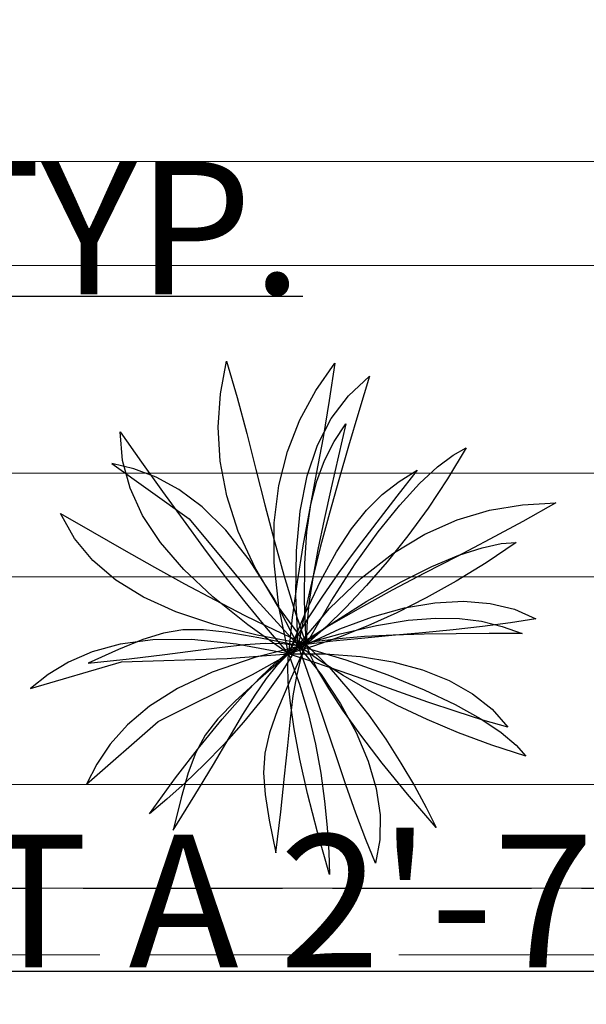
# Model space of a CAD drawing. Units: inches. Extents: x 351 to 1738, y -265 to 286.
# Tile 12 of 38: x 1142 to 1176, y -206 to -147. Entities that reach past the tile are written whole.
import ezdxf

# ---------------------------------------------------------------- set-up
doc = ezdxf.new("R2010")
doc.units = ezdxf.units.IN
doc.header["$MEASUREMENT"] = 0
doc.linetypes.add('ACAD_ISO02W100', pattern=[15, 12, -3])
for name, color, linetype, lineweight in [('A-ANNO-DIMS', 2, 'Continuous', 18), ('A-FLOR-OVHD', 1, 'ACAD_ISO02W100', 18), ('A-FLOR-PATT', 9, 'Continuous', 9)]:
    doc.layers.add(name, color=color, linetype=linetype, lineweight=lineweight)
doc.layers.add('CAY', color=94, linetype='Continuous')
doc.layers.add('DIENHOA', color=3, linetype='Continuous')
doc.styles.get("Standard").update_dxf_attribs({"font": 'arial.ttf'})
doc.dimstyles.get("Standard").update_dxf_attribs({"dimtxt": 8, "dimasz": 5, "dimexe": 0.18, "dimexo": 0.0625, "dimgap": 0.09, "dimtad": 1, "dimtoh": 1, "dimzin": 0, "dimdsep": 46, "dimlunit": 4, "dimtxsty": 'Standard', "dimcen": 0, "dimclre": 256, "dimadec": 0, "dimazin": 0, "dimtfac": 1, "dimtofl": 0, "dimtmove": 0, "dimatfit": 3, "dimfxl": 1, "dimtolj": 1, "dimtzin": 0, "dimlwe": -1, "dimarcsym": 0})

# ---------------------------------------------------------------- blocks, each defined once
blk = doc.blocks.new('Cay03_mb')
at = {"layer": 'DIENHOA'}
for p, q in [((118.6, 555.3), (166.2, 599.1)), ((166.2, 599.1), (142.2, 519.4)), ((79.5, 503.7), (118.6, 555.3)), ((142.2, 519.4), (119, 441.7)), ((48.6, 443.6), (79.5, 503.7)), ((25.5, 374.3), (48.6, 443.6)), ((119, 441.7), (96.7, 365.6)), ((-365.2, 390.3), (-414.4, 402.8)), ((-414.4, 402.8), (-240.2, 277.8)), ((-314.9, 371.3), (-365.2, 390.3)), ((-263.5, 343.5), (-314.9, 371.3)), ((9.9, 295.3), (25.5, 374.3)), ((96.7, 365.6), (75.6, 290.6)), ((-211.2, 304.6), (-263.5, 343.5)), ((511, 309.6), (585.9, 313.5)), ((585.9, 313.5), (511.8, 271.4)), ((-158, 252.3), (-211.2, 304.6)), ((1.6, 205.7), (9.9, 295.3)), ((75.6, 290.6), (55.7, 216.3)), ((363.4, 275.4), (436.8, 297.2)), ((436.8, 297.2), (511, 309.6)), ((-240.2, 277.8), (-88.4, 94.9)), ((290.6, 243.2), (363.4, 275.4)), ((511.8, 271.4), (437.6, 231.5)), ((-104.2, 184.4), (-158, 252.3)), ((218.5, 199.8), (290.6, 243.2)), ((437.6, 231.5), (363.7, 192.9)), ((0.2, 104.9), (1.6, 205.7)), ((55.7, 216.3), (37.3, 142.1)), ((-49.6, 98.5), (-104.2, 184.4)), ((147, 144.1), (218.5, 199.8)), ((363.7, 192.9), (290.2, 154.9)), ((37.3, 142.1), (20.5, 67.6)), ((75.9, 75.2), (147, 144.1)), ((290.2, 154.9), (217.4, 116.6)), ((217.4, 116.6), (145.5, 77.3)), ((-88.4, 94.9), (5.4, -7.8)), ((5.4, -7.8), (-49.6, 98.5)), ((5.4, -7.8), (0.2, 104.9)), ((5.4, -7.8), (75.9, 75.2)), ((20.5, 67.6), (5.4, -7.8)), ((145.5, 77.3), (74.7, 36.1)), ((182.2, 37.2), (253, 48.9)), ((253, 48.9), (314.6, 54.1)), ((314.6, 54.1), (369.2, 53.3)), ((369.2, 53.3), (418.6, 46.8)), ((418.6, 46.8), (464.9, 35.2)), ((-254.7, 27.4), (-298.6, 20.1)), ((-208, 27.8), (-254.7, 27.4)), ((-152.7, 21.7), (-208, 27.8)), ((74.7, 36.1), (5.4, -7.8)), ((100.3, 18.4), (182.2, 37.2)), ((464.9, 35.2), (510, 19)), ((-345, 5.4), (-399.6, -17.1)), ((-298.6, 20.1), (-345, 5.4)), ((-83.4, 9.7), (-152.7, 21.7)), ((5.4, -7.8), (-83.4, 9.7)), ((5.4, -7.8), (100.3, 18.4)), ((46.3, 0.9), (5.4, -7.8)), ((96.7, 7.5), (46.3, 0.9)), ((155, 12.2), (96.7, 7.5)), ((219.6, 15.4), (155, 12.2)), ((289, 17.4), (219.6, 15.4)), ((361.6, 18.5), (289, 17.4)), ((435.8, 18.9), (361.6, 18.5)), ((510, 19), (435.8, 18.9)), ((-399.6, -17.1), (-468, -47.9)), ((-295.3, -27.9), (-225.8, -18.9)), ((-225.8, -18.9), (-165.8, -11.3)), ((-165.8, -11.3), (-114, -5.7)), ((-114, -5.7), (-69, -2.9)), ((-69, -2.9), (-29.6, -3.4)), ((5.4, -7.8), (-33.2, -69.5)), ((-29.6, -3.4), (5.4, -7.8)), ((-16.5, -22.4), (5.4, -7.8)), ((5.4, -7.8), (56.8, -73.3)), ((25.9, -64.4), (5.4, -7.8)), ((5.4, -7.8), (112.8, -40.3)), ((53.5, -41.6), (5.4, -7.8)), ((-468, -47.9), (-375.6, -37.8)), ((-375.6, -37.8), (-295.3, -27.9)), ((-45.1, -46.3), (-16.5, -22.4)), ((107, -75.7), (53.5, -41.6)), ((112.8, -40.3), (207.5, -73.8)), ((-79.8, -79.6), (-45.1, -46.3)), ((47, -125.9), (25.9, -64.4)), ((-120.2, -122.1), (-79.8, -79.6)), ((-33.2, -69.5), (-74.6, -127.3)), ((56.8, -73.3), (100.4, -139.1)), ((165.5, -109.6), (107, -75.7)), ((207.5, -73.8), (289.5, -107.6)), ((228.7, -142.8), (165.5, -109.6)), ((289.5, -107.6), (359.3, -141.1)), ((-165.9, -174.1), (-120.2, -122.1)), ((-74.6, -127.3), (-117.8, -181.1)), ((68.7, -190.6), (47, -125.9)), ((100.4, -139.1), (135.9, -204.3)), ((296, -174.7), (228.7, -142.8)), ((359.3, -141.1), (416.9, -173.5)), ((-216.3, -235.6), (-165.9, -174.1)), ((367.1, -204.8), (296, -174.7)), ((416.9, -173.5), (462.6, -204.2)), ((-117.8, -181.1), (-162.1, -230.9)), ((90.8, -256.6), (68.7, -190.6)), ((135.9, -204.3), (162.8, -268.3)), ((441.6, -232.7), (367.1, -204.8)), ((462.6, -204.2), (496.5, -232.5)), ((-271, -306.6), (-216.3, -235.6)), ((-162.1, -230.9), (-206.3, -276.5)), ((518.9, -257.7), (441.6, -232.7)), ((496.5, -232.5), (518.9, -257.7)), ((113.1, -322.2), (90.8, -256.6)), ((-206.3, -276.5), (-249.6, -317.8)), ((162.8, -268.3), (181, -330.4)), ((-329.5, -387.1), (-271, -306.6)), ((-249.6, -317.8), (-291, -354.7)), ((135.4, -385.6), (113.1, -322.2)), ((181, -330.4), (190, -390)), ((-291, -354.7), (-329.5, -387.1)), ((157.6, -445), (135.4, -385.6)), ((190, -390), (189.6, -446.3)), ((179.5, -498.7), (157.6, -445)), ((189.6, -446.3), (179.5, -498.7))]:
    blk.add_line(p, q, dxfattribs=at)
for points in [[(23.7, -5.4), (-41, 82.2), (-91.8, 167.1), (-129.7, 249.5), (-155.6, 329.6), (-170.2, 407.8), (-174.7, 484.2), (-169.8, 559.3), (-156.5, 633.1)], [(-156.5, 633.1), (-132.5, 551.3), (-110.5, 470), (-89.8, 389.2), (-69.6, 309), (-49, 229.4), (-27.1, 150.4), (-3.2, 72.1), (23.7, -5.4)], [(-16.4, -26.7), (-38.3, 80), (-48.9, 178.3), (-48.7, 269), (-38.5, 352.6), (-19.1, 429.7), (9, 501), (44.9, 567.1), (87.9, 628.5)], [(87.9, 628.5), (75.5, 544.2), (61.3, 461.2), (46.1, 379.1), (30.8, 297.8), (16.1, 216.9), (2.9, 136), (-8.3, 54.9), (-16.4, -26.7)], [(23.7, -5.4), (19.8, 93), (20.3, 177), (25, 248.5), (34, 309.8), (47.3, 362.7), (64.9, 409.3), (86.8, 451.7), (112.9, 491.9)], [(112.9, 491.9), (96, 419.7), (79.5, 347.4), (63.9, 276.5), (50, 208.4), (38.4, 144.8), (29.7, 86.9), (24.6, 36.3), (23.7, -5.4)], [(-395.6, 473.7), (-347.5, 405.6), (-300.6, 339.5), (-254.3, 275.1), (-208.3, 212.3), (-161.9, 150.9), (-114.8, 90.7), (-66.5, 31.6), (-16.4, -26.7)], [(-16.4, -26.7), (-108.3, 38.6), (-186.9, 101.7), (-252.4, 163.5), (-305.1, 224.4), (-345.4, 285.2), (-373.7, 346.6), (-390.4, 409.2), (-395.6, 473.7)], [(384.3, 437.5), (342.2, 367.8), (298.1, 301.7), (252.6, 239.4), (206.1, 181.1), (159.4, 127.2), (113, 78), (67.6, 33.6), (23.7, -5.4)], [(23.7, -5.4), (79.9, 91.7), (134.1, 176.2), (185.8, 248.4), (234.3, 308.7), (279, 357.3), (319.3, 394.8), (354.6, 421.4), (384.3, 437.5)], [(273.2, 387.3), (227.6, 328.8), (182.3, 270.1), (138.4, 212.3), (97.2, 156.4), (60, 103.4), (27.8, 54.6), (1.9, 10.8), (-16.4, -26.7)], [(-16.4, -26.7), (21.4, 64.2), (57, 140.3), (91.4, 203.3), (125.2, 255.1), (159.5, 297.5), (195, 332.5), (232.7, 361.8), (273.2, 387.3)], [(-530.5, 289.7), (-458.3, 248.1), (-387.9, 207.8), (-318.9, 168.7), (-250.8, 131.1), (-182.9, 94.8), (-114.9, 59.9), (-46.2, 26.5), (23.7, -5.4)], [(23.7, -5.4), (-87.2, 15.2), (-185, 39.6), (-270.3, 68.2), (-343.7, 101.4), (-405.9, 139.7), (-457.3, 183.5), (-498.7, 233.4), (-530.5, 289.7)], [(496.7, 224), (429.4, 178.4), (361.6, 136.9), (294.1, 99.5), (227.5, 66.1), (162.4, 36.7), (99.7, 11.5), (39.8, -9.7), (-16.4, -26.7)], [(-16.4, -26.7), (75.4, 37.9), (160.1, 91.8), (237.3, 135.7), (306.6, 170), (367.6, 195.4), (419.9, 212.5), (463.1, 221.9), (496.7, 224)], [(23.7, -5.4), (99.3, 29.7), (173.2, 57.1), (244.8, 76.7), (313.3, 88.3), (377.9, 91.8), (437.9, 87), (492.7, 73.8), (541.4, 52)], [(541.4, 52), (484.1, 42.9), (421.2, 34.8), (354.4, 27.6), (285.4, 20.9), (216.1, 14.5), (148.2, 8.1), (83.5, 1.6), (23.7, -5.4)], [(-16.4, -26.7), (-134, -4.7), (-235.3, 5.3), (-322, 4.7), (-395.9, -5), (-458.7, -22.3), (-512.3, -45.7), (-558.2, -73.6), (-598.4, -104.7)], [(-471.9, -320.3), (-310.5, -179.3), (-97.7, -73.3), (23.7, -5.4)], [(23.7, -5.4), (-92.3, -34.8), (-188.4, -68.2), (-266.9, -105.1), (-329.9, -144.9), (-379.7, -187), (-418.5, -230.7), (-448.5, -275.3), (-471.9, -320.3)], [(23.7, -5.4), (-13.6, -87.9), (-41.1, -152.6), (-59.6, -205), (-69.9, -250.7), (-72.8, -295), (-69.2, -343.6), (-59.7, -401.9), (-45.3, -475.5)], [(-45.3, -475.5), (-34.1, -383.2), (-25.4, -302.8), (-18.3, -233.1), (-12, -172.9), (-5.6, -121.2), (2, -76.8), (11.4, -38.5), (23.7, -5.4)], [(316.5, -418.1), (251.4, -342.8), (194.8, -273.3), (146.5, -210.2), (106.3, -153.8), (74.1, -104.7), (49.7, -63.4), (32.9, -30.1), (23.7, -5.4)], [(23.7, -5.4), (74.9, -57.1), (121.8, -110.6), (164.3, -165), (202.7, -219.4), (237, -272.9), (267.3, -324.5), (293.7, -373.2), (316.5, -418.1)], [(-598.4, -104.7), (-392.7, -44.4), (-155, -37.4), (-16.4, -26.7)], [(-276.2, -424.4), (-227.3, -345.4), (-185.7, -276.1), (-150, -215.7), (-119.1, -163.8), (-91.5, -119.5), (-66, -82.3), (-41.4, -51.6), (-16.4, -26.7)], [(-16.4, -26.7), (-84.9, -86), (-137, -133.1), (-175.8, -173), (-204.3, -210), (-225.5, -249.1), (-242.5, -294.7), (-258.4, -351.6), (-276.2, -424.4)], [(76.2, -524.2), (48.8, -428.5), (26.6, -341.7), (9.2, -264.1), (-3.6, -196.1), (-12.3, -138), (-17.1, -90.2), (-18.3, -53), (-16.4, -26.7)], [(-16.4, -26.7), (66.9, -26.6), (145.6, -32.7), (218.8, -44.9), (285.8, -63.1), (345.9, -87.1), (398.4, -116.6), (442.6, -151.6), (477.6, -191.8)], [(477.6, -191.8), (421.8, -176), (361.3, -156.9), (297.6, -135.5), (232.2, -112.6), (166.6, -89.4), (102.3, -66.6), (40.8, -45.4), (-16.4, -26.7)], [(-16.4, -26.7), (8.5, -95.1), (28.5, -163.3), (44.3, -230.6), (56.3, -296.1), (65, -359), (70.9, -418.5), (74.5, -473.9), (76.2, -524.2)]]:
    blk.add_lwpolyline(points, dxfattribs=at)
blk = doc.blocks.new('*D36')
at = {"layer": 'A-ANNO-DIMS', "transparency": 16777216}
for p, q in [((1073.569, -199.341), (1073.569, -204.202)), ((1105.198, -199.341), (1105.198, -204.202))]:
    blk.add_line(p, q, dxfattribs=at)
at = {"layer": 'A-ANNO-DIMS', "color": 0, "lineweight": -2, "transparency": 16777216}
for p, q in [((1078.569, -204.022), (1100.198, -204.022)), ((1105.198, -204.022), (1227.071, -204.022))]:
    blk.add_line(p, q, dxfattribs=at)
at = {"layer": 'A-ANNO-DIMS', "color": 0, "transparency": 16777216}
for points in [[(1078.569, -203.189), (1078.569, -204.856), (1073.569, -204.022)], [(1100.198, -203.189), (1100.198, -204.856), (1105.198, -204.022)]]:
    blk.add_solid(points, dxfattribs=at)
at = {"layer": 'Defpoints', "color": 0, "transparency": 16777216}
for p in [(1073.569, -199.278), (1105.198, -199.278), (1105.198, -204.022)]:
    blk.add_point(p, dxfattribs=at)
at = {"layer": 'A-ANNO-DIMS', "color": 0, "transparency": 16777216, "insert": (1168.634, -199.796), "char_height": 8, "attachment_point": 5}
blk.add_mtext('\\A1;PLANT A 2\'-7 1/2" TYP.', dxfattribs=at)
blk = doc.blocks.new('*D37')
at = {"layer": 'A-ANNO-DIMS', "color": 0, "lineweight": -2, "transparency": 16777216}
for p, q in [((1109.942, -168.369), (1109.942, -163.369)), ((1109.942, -163.369), (1158.933, -163.369)), ((1109.942, -194.278), (1109.942, -173.369))]:
    blk.add_line(p, q, dxfattribs=at)
at = {"layer": 'A-ANNO-DIMS', "transparency": 16777216}
for p, q in [((1105.26, -168.369), (1110.122, -168.369)), ((1105.26, -199.278), (1110.122, -199.278))]:
    blk.add_line(p, q, dxfattribs=at)
at = {"layer": 'A-ANNO-DIMS', "color": 0, "transparency": 16777216}
for points in [[(1109.109, -173.369), (1110.775, -173.369), (1109.942, -168.369)], [(1109.109, -194.278), (1110.775, -194.278), (1109.942, -199.278)]]:
    blk.add_solid(points, dxfattribs=at)
at = {"layer": 'Defpoints', "color": 0, "transparency": 16777216}
for p in [(1105.198, -168.369), (1109.942, -168.369), (1105.198, -199.278)]:
    blk.add_point(p, dxfattribs=at)
at = {"layer": 'A-ANNO-DIMS', "color": 0, "transparency": 16777216, "insert": (1134.482, -159.26), "char_height": 8, "attachment_point": 5}
blk.add_mtext('\\A1;2\'-7" TYP.', dxfattribs=at)

msp = doc.modelspace()

# ---------------------------------------------------------------- hatches: boundary and pattern name
at = {"layer": 'A-FLOR-PATT', "transparency": 33554559}
h = msp.add_hatch(dxfattribs=at)
h.set_pattern_fill('ANSI37', color=256, scale=200, angle=135)
h.set_pattern_definition([(180, (1112.704, -164.037), (-2e-15, -25), []), (270, (1112.704, -164.037), (25, -5e-15), [])])
h.paths.add_polyline_path([(1380.064, 73.463), (1380.132, 148.463), (1338.064, 148.463), (1290.704, 148.463), (1290.704, 88.463), (1248.704, 88.463), (1248.704, -2.009), (1244.704, -2.009), (1244.704, 142.457), (1160.704, 142.457), (1160.704, 158.963), (1160.704, 170.137), (1160.704, 206.137), (1160.704, 228.963), (1112.704, 228.963), (1112.704, 209.963), (1112.704, 168.963), (1124.704, 168.963), (1124.704, 162.963), (1112.704, 162.963), (1112.704, 64.463), (1112.704, 60.463), (1112.704, 0.463), (1112.704, -48.026), (1146.804, -47.981), (1146.804, -35.691), (1207.804, -35.691), (1207.804, -47.902), (1236.542, -47.864), (1236.544, -50.009), (1248.5, -50.009), (1248.506, -102.915), (1248.512, -150.915), (1248.514, -164.037), (1248.549, -164.037), (1273.017, -164.037), (1273.017, -128.799), (1355.24, -128.799), (1355.24, -164.037), (1384.204, -164.037), (1384.204, -57.037), (1380.064, -57.037), (1380.064, -48.037), (1392.064, -48.037), (1392.064, -53.037), (1406.549, -53.037), (1406.549, -57.037), (1401.204, -57.037), (1401.204, -147.037), (1468.204, -147.037), (1468.204, -138.5), (1472.204, -138.5), (1472.204, -102.5), (1468.204, -102.5), (1468.204, -57.037), (1442.549, -57.037), (1442.549, -53.037), (1463.049, -53.037), (1463.049, -40.747), (1524.049, -40.747), (1524.049, -48.037), (1536.064, -48.037), (1536.064, -53.037), (1557.704, -53.037), (1557.704, 204.963), (1384.204, 204.963), (1384.204, 73.463), (1392.064, 73.463), (1392.064, 64.463), (1384.204, 64.463), (1384.204, -3.5), (1380.204, -3.537), (1380.204, 64.463), (1380.064, 64.463)])
h.paths.add_polyline_path([(1510.714, 86.458, -0.103984), (1511.661, 85.595, 0.470438), (1510.158, 87.614, 0.0961)], flags=16)
h.paths.add_polyline_path([(1510.443, 100.266, 0.009798), (1504.693, 100.48, 0.02879), (1504.6, 99.767, -0.165331), (1505.519, 96.135, -0.143601)], flags=16)
h.paths.add_polyline_path([(1487.201, 85.595, -0.103984), (1488.148, 86.458, 0.0961), (1488.704, 87.614, 0.470438)], flags=0)
h.paths.add_polyline_path([(1495.052, 100.43), (1494.178, 100.43, -0.026463), (1494.262, 99.774, -0.144219)], flags=16)
h.paths.add_polyline_path([(1444.485, 86.458, -0.103984), (1445.433, 85.595, 0.470438), (1443.93, 87.614, 0.0961)], flags=16)
h.paths.add_polyline_path([(1420.972, 85.595, -0.103984), (1421.92, 86.458, 0.0961), (1422.475, 87.614, 0.470438)], flags=16)
h.paths.add_polyline_path([(1428.632, 100.335, 0.001054), (1427.971, 100.309, -0.021524), (1428.033, 99.774, -0.114301)], flags=16)
h.paths.add_polyline_path([(1419.906, 143.708, 0.024979), (1420.222, 157.526), (1421.573, 159.101), (1421.573, 175.369), (1391.393, 175.369), (1391.393, 200.519), (1542.294, 200.519), (1542.294, 175.369), (1512.028, 175.369, 0.019865), (1511.521, 153.838, 0.025134), (1512.758, 118.323, 0.020553), (1512.942, 115.253), (1419.834, 115.253, -0.000414), (1419.843, 124.798), (1413.059, 124.798), (1413.059, 84.437, -0.061853), (1415.831, 80.45, -0.093077), (1420.972, 85.595, -0.267537), (1422.371, 84.732, 0.08511), (1424.052, 84.616, -0.885393), (1424.033, 84.851, -1.125815), (1424.073, 84.366, -0.087987), (1422.371, 84.732, -0.267537), (1422.326, 83.089, -0.370542), (1420.972, 85.595, 0.093077), (1415.831, 80.45, -0.087414), (1417.914, 73.937), (1418.941, 73.937, 0.02725), (1418.913, 76.906, -0.115703), (1421.051, 73.937), (1445.354, 73.937, -0.115703), (1447.492, 76.906, 0.02725), (1447.464, 73.937), (1448.491, 73.937, -0.087414), (1450.574, 80.45, 0.093077), (1445.433, 85.595, -0.370542), (1444.079, 83.089, -0.267537), (1444.034, 84.732, -0.087987), (1442.332, 84.366, -1.125815), (1442.372, 84.851, -2.032736), (1442.364, 84.368, 0.086378), (1444.034, 84.732, -0.267537), (1445.433, 85.595, -0.093077), (1450.574, 80.45, -0.257732), (1466.483, 90.927, -0.47867), (1468.832, 91.907, -0.47867), (1471.18, 90.927, -0.26264), (1483.053, 81.78, -0.071866), (1487.201, 85.595, -0.267537), (1488.6, 84.732, 0.08511), (1490.28, 84.616, -0.885393), (1490.262, 84.851, -1.125815), (1490.301, 84.366, -0.087987), (1488.6, 84.732, -0.267537), (1488.554, 83.089, -0.370542), (1487.201, 85.595, 0.071866), (1483.053, 81.78, -0.132065), (1484.143, 73.937), (1485.169, 73.937, 0.02725), (1485.142, 76.906, -0.115703), (1487.28, 73.937), (1511.582, 73.937, -0.115703), (1513.72, 76.906, 0.02725), (1513.693, 73.937), (1514.719, 73.937, -0.087414), (1516.802, 80.45, 0.093077), (1511.661, 85.595, -0.370542), (1510.308, 83.089, -0.267537), (1510.262, 84.732, -0.087987), (1508.561, 84.366, -1.125815), (1508.601, 84.851, -2.032736), (1508.592, 84.368, 0.086378), (1510.262, 84.732, -0.267537), (1511.661, 85.595, -0.093077), (1516.802, 80.45, -0.061853), (1519.575, 84.437), (1519.575, 73.937), (1413.059, 73.937), (1413.059, 124.798), (1419.843, 124.798, -0.000821)], flags=16)
h.paths.add_polyline_path([(1220.149, 54.133, -0.103984), (1220.869, 53.476, 0.470438), (1219.727, 55.011, 0.0961)], flags=16)
h.paths.add_polyline_path([(1219.944, 64.626, 0.009798), (1215.574, 64.789, 0.02879), (1215.503, 64.247, -0.165331), (1216.201, 61.487, -0.143601)], flags=16)
h.paths.add_polyline_path([(1209.779, 64.449, 0.097446), (1209.339, 64.751), (1208.247, 64.751, 0.12739), (1207.7, 64.326, 0.171586), (1206.95, 61.475, -0.158854), (1207.636, 59.45, 0.015898), (1207.795, 59.218, 0.061546), (1208.598, 59.616, 0.175416), (1208.638, 60.099, -0.284779), (1209.348, 62.472, 0.326216)], flags=16)
h.paths.add_polyline_path([(1169.818, 54.133, -0.103984), (1170.538, 53.476, 0.470438), (1169.396, 55.011, 0.0961)], flags=16)
h.paths.add_polyline_path([(1159.017, 62.472, 0.284764), (1158.307, 60.099, -0.175433), (1158.267, 59.616, 0.39293), (1159.448, 64.449, -0.32623)], flags=16)
h.paths.add_polyline_path([(1156.342, 58.239, -0.178321), (1154.011, 55.31, -0.174736), (1154.722, 55.233, -0.200802), (1156.27, 56.086, 0.12699), (1157.283, 58.991, -0.091205)], flags=16)
h.paths.add_polyline_path([(1156.624, 61.413, 0.157275), (1157.316, 64.247, 0.169622)], flags=16)
h.paths.add_polyline_path([(1152.67, 54.133, -0.0961), (1151.95, 53.476, 0.064076), (1154.465, 54.384, 0.199016)], flags=16)
h.paths.add_polyline_path([(1202.281, 53.476, -0.103984), (1203, 54.133, 0.0961), (1203.423, 55.011, 0.470438)], flags=0)
h.paths.add_polyline_path([(1151.139, 97.64, 0.024979), (1151.379, 108.141), (1152.406, 109.338), (1152.406, 121.701), (1129.47, 121.701), (1129.47, 140.814), (1244.149, 140.814), (1244.149, 121.701), (1221.148, 121.701, 0.019865), (1220.763, 105.338, 0.025134), (1221.703, 78.349, 0.020553), (1221.843, 76.016), (1151.078, 76.016, -0.128743), (1148.786, 65.037, 0.539352), (1150.327, 64.171, -0.027594), (1163.481, 64.751, 0.097695), (1163.04, 64.449, 0.326216), (1163.471, 62.472, -0.284777), (1164.181, 60.099, -0.194757), (1165.846, 61.443, -0.155402), (1165.172, 64.247, -0.166022), (1165.869, 61.475, -0.177014), (1167.852, 62.77, -0.448203), (1169.974, 60.807, -0.393499), (1167.679, 57.86, -0.895548), (1168.438, 54.524, -0.355767), (1166.218, 56.086, -0.066024), (1165.505, 57.539), (1165.251, 56.243, -0.371732), (1164.02, 59.758, -0.373614), (1163.04, 64.449, -0.097695), (1163.481, 64.751, 0.021354), (1153.294, 64.429, -0.134183), (1156.695, 61.368, 0.186873), (1154.636, 62.77, 0.448203), (1152.514, 60.807, 0.403726), (1154.905, 57.846, 0.711219), (1153.334, 55, 0.53154), (1151.95, 53.476, -0.267537), (1153.013, 52.821, 0.08511), (1154.29, 52.732, -0.885393), (1154.276, 52.911, -1.125815), (1154.306, 52.543, -0.087987), (1153.013, 52.821, -0.267537), (1152.978, 51.572, -0.370542), (1151.95, 53.476, 0.093077), (1148.043, 49.566, -0.087414), (1149.626, 44.617), (1150.406, 44.617, 0.02725), (1150.385, 46.873, -0.115703), (1152.01, 44.617), (1170.478, 44.617, -0.115703), (1172.103, 46.873, 0.02725), (1172.082, 44.617), (1172.862, 44.617, -0.087414), (1174.445, 49.566, 0.093077), (1170.538, 53.476, -0.370542), (1169.51, 51.572, -0.267537), (1169.475, 52.821, -0.087987), (1168.182, 52.543, -1.125815), (1168.212, 52.911, -2.032736), (1168.206, 52.544, 0.086378), (1169.475, 52.821, -0.267537), (1170.538, 53.476, -0.093077), (1174.445, 49.566, -0.257732), (1186.536, 57.528, -0.47867), (1188.321, 58.273, -0.47867), (1190.106, 57.528, -0.26264), (1199.128, 50.577, -0.071866), (1202.281, 53.476, -0.267537), (1203.344, 52.821, 0.08511), (1204.621, 52.732, -0.885393), (1204.607, 52.911, -1.125815), (1204.637, 52.543, -0.087987), (1203.344, 52.821, -0.267537), (1203.309, 51.572, -0.370542), (1202.281, 53.476, 0.071866), (1199.128, 50.577, -0.132065), (1199.957, 44.617), (1200.737, 44.617, 0.02725), (1200.716, 46.873, -0.115703), (1202.341, 44.617), (1220.809, 44.617, -0.115703), (1222.434, 46.873, 0.02725), (1222.413, 44.617), (1223.193, 44.617, -0.087414), (1224.776, 49.566, 0.093077), (1220.869, 53.476, -0.370542), (1219.841, 51.572, -0.267537), (1219.806, 52.821, -0.087987), (1218.513, 52.543, -1.125815), (1218.543, 52.911, -2.032736), (1218.537, 52.544, 0.086378), (1219.806, 52.821, -0.267537), (1220.869, 53.476, -0.093077), (1224.776, 49.566, -0.061853), (1226.883, 52.597), (1226.883, 44.617), (1145.936, 44.617), (1145.936, 83.269), (1151.091, 83.269, -0.000821)], flags=16)
h.paths.add_polyline_path([(1218.01, 57.86, -0.895548), (1218.769, 54.524, -0.355767), (1216.549, 56.086, -0.066024), (1215.836, 57.539), (1215.582, 56.243, -0.371732), (1214.351, 59.758, -0.373614), (1213.371, 64.449, 0.326216), (1213.802, 62.472, -0.284777), (1214.512, 60.099, -0.194757), (1216.177, 61.443, -0.179991), (1218.183, 62.77, -0.448203), (1220.305, 60.807, -0.393499)], flags=16)
h.paths.add_polyline_path([(1424.735, 91.363, -0.393499), (1421.715, 95.241, -0.448203), (1424.507, 97.824, -0.179991), (1427.147, 96.077, -0.194757), (1429.338, 94.309, -0.284777), (1430.272, 97.432, 0.326216), (1430.839, 100.034, -0.373614), (1429.55, 93.861, -0.371732), (1427.929, 89.235), (1427.596, 90.941, -0.066024), (1426.657, 89.029, -0.355767), (1423.736, 86.973, -0.895548)], flags=16)
h.paths.add_polyline_path([(1238.033, 131.257, -1), (1227.329, 131.257, -1)], flags=0)
h.paths.add_polyline_path([(1235.357, 131.257, -1), (1230.005, 131.257, -1)], flags=0)
h.paths.add_polyline_path([(1214.039, 54.243, 0.154382), (1214.38, 53.992, 0.358955), (1213.613, 54.016, 0.603948), (1214.379, 53.657, 0.371319), (1213.968, 52.872, 0.187994), (1214.312, 52.809, -0.592455), (1213.953, 52.967, -0.294279), (1214.083, 53.691, -1.300187), (1213.881, 54.134, -0.283762), (1214.469, 53.896, 1.15094)], flags=16)
h.paths.add_polyline_path([(1212.091, 56.286, -0.408434), (1211.337, 56.445, -0.036259), (1211.098, 56.848, -0.236098), (1211.59, 56.63, 0.035345), (1211.835, 56.543, -0.475241), (1212.091, 56.286, -0.475241), (1212.438, 56.182, 0.035345), (1212.631, 56.007, -0.236098), (1213.056, 55.676, -0.036259), (1212.588, 55.697, -0.408434)], flags=16)
h.paths.add_polyline_path([(1211.469, 50.297, 0.296043), (1210.47, 50.527, 0.310883), (1211.931, 50.148, 0.021255)], flags=16)
h.paths.add_polyline_path([(1213.739, 51.818, -0.036259), (1213.271, 51.838, -0.408434), (1212.774, 52.427, -0.094786), (1212.293, 50.703, 1.150474), (1212.911, 50.232, 0.166288), (1213.265, 50.68, -0.025254), (1212.603, 50.13, 1.087932), (1212.471, 49.407, 0.166288), (1213.02, 49.251, -0.016128), (1212.567, 49.563, -0.286859), (1212.217, 49.638, 0.022156), (1212.046, 50.055, -0.64613), (1212.185, 50.498, 0.088412), (1212.732, 52.077, -1.186037), (1213.121, 52.323, 0.035345), (1213.314, 52.148, -0.236098)], flags=16)
h.paths.add_polyline_path([(1212.094, 50.342, -0.048524), (1211.54, 49.605, -1.103834), (1211.397, 48.738, -0.785515), (1211.683, 48.254, -0.392043), (1210.948, 48.525, -0.392819), (1210.561, 47.995, -0.592455), (1210.201, 48.153, -0.294279), (1210.331, 48.877, -0.704172), (1210.316, 49.592, -0.679344), (1210.729, 50.112, 0.563676)], flags=16)
h.paths.add_polyline_path([(1211.274, 49.829, -0.139826), (1210.745, 49.859, -0.217879), (1210.948, 49.509, -0.498572)], flags=0)
h.paths.add_polyline_path([(1433.426, 81.49, -0.181571), (1434.245, 81.788, -0.008067), (1433.726, 82.205, 0.045578), (1432.755, 81.242, 0.179011)], flags=16)
h.paths.add_polyline_path([(1434.146, 81.009, -0.132442), (1433.645, 80.771, 0.259089), (1433.234, 80.471, -0.180211), (1433.392, 80.805, -0.16994), (1432.758, 81.109, 0.032652), (1433.273, 80.474, -0.493363), (1434.046, 80.146, -0.390497)], flags=16)
h.paths.add_polyline_path([(1434.83, 80.047, -0.947538), (1435.294, 79.576, -0.299128), (1434.625, 79.404, -0.270439), (1435.01, 78.591, -0.592455), (1434.537, 78.382, -0.392819), (1434.027, 79.08, -0.392043), (1433.06, 78.723, -0.352042), (1433.003, 79.197, -0.197216), (1433.75, 79.734, -0.71364), (1434.447, 79.939, -0.21479), (1434.819, 80.475, 0.408833), (1435.075, 80.803, -0.226152)], flags=16)
h.paths.add_polyline_path([(1432.67, 81.217, -0.454218), (1431.897, 79.923, -0.414411), (1431.301, 80.035, 0.016129), (1431.897, 80.445, 0.27957), (1432.073, 80.871, -0.289504), (1431.103, 81.321, -0.414411), (1430.978, 81.915, 0.01613), (1431.586, 81.521, 0.341293), (1432.125, 81.583, -0.813186)], flags=16)
h.paths.add_polyline_path([(1429.893, 86.381, -0.947538), (1430.358, 85.91, -0.173106), (1429.984, 85.712, -0.038817), (1431.625, 84.214, -0.0879), (1432.097, 88.549, -0.049768), (1431.254, 88.49, -0.236098), (1431.814, 88.925, 0.035345), (1432.067, 89.155, -0.475241), (1432.524, 89.291, -0.475241), (1432.86, 89.63, 0.035345), (1433.182, 89.744, -0.236098), (1433.83, 90.032, -0.036259), (1433.516, 89.502, -0.408434), (1432.524, 89.291, -0.312424), (1432.106, 88.58, 0.088559), (1431.625, 84.214, -0.408434), (1430.971, 83.439, -0.036259), (1430.355, 83.412, -0.236098), (1430.914, 83.847, 0.035345), (1431.168, 84.078, -0.475241), (1431.625, 84.214, 0.038817), (1429.984, 85.712, -0.321732), (1429.333, 86.048, -0.32743), (1429.883, 86.809, 0.408833), (1430.138, 87.138, -0.226152)], flags=16)
h.paths.add_polyline_path([(1211.206, 58.616, -0.999784), (1211.336, 59.323, -0.614994)], flags=16)
h.paths.add_polyline_path([(1210.288, 49.429, 0.154382), (1210.629, 49.178, 0.358955), (1209.861, 49.202, 0.603948), (1210.627, 48.843, -0.534825), (1210.806, 49.295, 0.748346)], flags=16)
h.paths.add_polyline_path([(1209.589, 51.828, -0.008791), (1209.775, 51.753, 0.112231), (1209.466, 52.019, 1.418851), (1209.014, 51.708, -0.458726), (1208.651, 51.073, -0.592455), (1208.291, 51.232, -0.294279), (1208.421, 51.955, -1.300187), (1208.219, 52.398, -0.226005), (1208.719, 52.257, -0.475519), (1209.158, 52.369, -1.455499), (1209.603, 52.664, 0.421305), (1209.191, 52.262, -0.591212), (1208.979, 51.796, 0.497399), (1209.773, 51.333, 0.649312)], flags=16)
h.paths.add_polyline_path([(1208.029, 52.041, 0.544667), (1208.832, 52.045, 0.220132)], flags=0)
h.paths.add_polyline_path([(1210.438, 51.425, -0.2042), (1210.277, 52.018, 0.270826), (1209.915, 52.897, 0.324115)], flags=0)
h.paths.add_polyline_path([(1209.668, 52.407, -0.60139), (1208.99, 52.221, -0.394916), (1208.248, 52.83, -0.836792), (1208.651, 53.017, -0.338488), (1209.039, 52.571, 0.194138), (1209.191, 52.262, 0.413995), (1209.712, 52.475, 0.51771), (1210.503, 51.416, 0.401922), (1209.493, 50.93, 0.206396), (1209.516, 50.165, -0.319463), (1210.417, 51.418, -0.466635)], flags=16)
h.paths.add_polyline_path([(1206.601, 56.086, -0.355767), (1204.381, 54.524, -0.921198), (1205.236, 57.846, 0.206569), (1207.614, 58.991, -0.12699)], flags=16)
h.paths.add_polyline_path([(1435.487, 82.816, 0.527765), (1436.615, 83.361, 0.50854), (1437.05, 82.433, 0.592455), (1437.524, 82.641, 0.331245), (1436.963, 83.548, 0.387863), (1437.808, 83.626, 0.592954), (1437.618, 84.176, 0.226016), (1436.961, 83.99, 0.318205), (1437.588, 84.854, 0.689374), (1437.05, 84.991, 0.335765), (1436.539, 84.41, -0.156993), (1436.404, 84.065, -0.434611), (1436.961, 83.99, -0.21479), (1437.333, 84.526, 0.408833), (1437.588, 84.854, -0.226152), (1437.343, 84.097, -0.947538), (1437.808, 83.626, -0.299128), (1437.139, 83.455, -0.270439), (1437.524, 82.641, -0.592455), (1437.05, 82.433, -0.392819), (1436.541, 83.13, -0.43966), (1435.475, 82.794, -0.174614), (1435.942, 82.244, -0.206396), (1435.912, 81.237, -0.270826), (1435.125, 82.208, 0.207976), (1434.686, 82.904, -0.196495)], flags=16)
h.paths.add_polyline_path([(1435.386, 84.832, 0.270811), (1434.91, 83.676, -0.204217), (1434.699, 82.895, 0.324115)], flags=0)
h.paths.add_polyline_path([(1435.68, 84.18, -0.217656), (1435.554, 83.304, -0.176705), (1436.236, 83.778, -0.373036)], flags=0)
h.paths.add_polyline_path([(1435.566, 100.034, 0.326216), (1436.133, 97.432, -0.284777), (1437.067, 94.309, -0.194757), (1439.258, 96.077, -0.155402), (1438.371, 99.767, -0.166022), (1439.289, 96.12, -0.177014), (1441.897, 97.824, -0.448203), (1444.69, 95.241, -0.393499), (1441.67, 91.363, -0.895548), (1442.669, 86.973, -0.355767), (1439.748, 89.029, -0.066024), (1438.809, 90.941), (1438.476, 89.235, -0.371732), (1436.855, 93.861, -0.373614)], flags=16)
h.paths.add_polyline_path([(1191.252, 49.507, -0.274022), (1190.658, 48.409, 0.267537), (1191.311, 47.344, 0.370542)], flags=0)
h.paths.add_polyline_path([(1190.301, 49.717, 0.199016), (1188.619, 49.04, 0.064076), (1191.252, 49.507, -0.0961)], flags=0)
h.paths.add_polyline_path([(1189.518, 47.857, 1.125815), (1189.676, 47.523, 2.044605)], flags=0)
h.paths.add_polyline_path([(1464.974, 80.372, 0.274022), (1465.756, 78.927, -0.083013)], flags=0)
h.paths.add_polyline_path([(1464.974, 80.372, 0.370542), (1464.897, 77.525, 0.576324)], flags=0)
h.paths.add_polyline_path([(1464.974, 80.372, -0.470438), (1467.284, 81.372, -0.0961), (1466.226, 80.648, -0.199016), (1468.439, 79.757, -0.064076)], flags=0)
h.paths.add_polyline_path([(1189.511, 56.43, -0.259467), (1188.321, 56.391, -0.259467), (1187.13, 56.43, 0.08511), (1188.193, 55.716, -0.885393), (1188.27, 55.878, -1.196013), (1188.355, 55.442, 0.101459)], flags=0)
h.paths.add_polyline_path([(1188.321, 57.596, 0.078072), (1187.678, 57.24, 0.01555), (1188.321, 57.136, 0.01555), (1188.964, 57.24, 0.078072)], flags=0)
h.paths.add_polyline_path([(1190.164, 55.365, -0.576324), (1190.106, 57.528, -0.198294), (1188.321, 58.319, -0.198294), (1186.536, 57.528, -0.576324), (1186.477, 55.365, -0.370542), (1186.536, 57.528, 0.198294), (1188.321, 58.319, 0.198294), (1190.106, 57.528, -0.370542)], flags=0)
h.paths.add_polyline_path([(1188.372, 55.878, 1.125814), (1188.529, 55.544, 2.044605)], flags=0)
h.paths.add_polyline_path([(1186.341, 49.717, -0.0961), (1185.389, 49.507, 0.064076), (1188.022, 49.04, 0.199016)], flags=0)
h.paths.add_polyline_path([(1185.389, 49.507, -0.267537), (1185.984, 48.409, 0.08511), (1187.046, 47.695, -0.885393), (1187.123, 47.857, -1.125815), (1186.966, 47.523, -0.087987), (1185.984, 48.409, -0.267537), (1185.331, 47.344, -0.370542)], flags=0)
h.paths.add_polyline_path([(1399.441, 187.944, -1), (1413.525, 187.944, -1)], flags=0)
h.paths.add_polyline_path([(1402.962, 187.944, -1), (1410.004, 187.944, -1)], flags=0)
h.paths.add_polyline_path([(1357.663, -72.245), (1377.272, -72.245), (1377.272, -91.854), (1357.663, -91.854)], flags=16)
h.paths.add_polyline_path([(1467.256, 78.201, -1.125815), (1467.049, 77.761, -2.044605)], flags=0)
h.paths.add_polyline_path([(1468.822, 88.714, 0.941125), (1469.106, 88.316, 1.137152), (1468.765, 88.755, 0.890986), (1468.99, 88.245, 0.094828), (1470.398, 89.481, -0.267537), (1471.18, 90.927, -0.028123), (1469.678, 90.547, -0.028774), (1469.948, 90.311, -0.020327), (1468.832, 90.41, -0.020327), (1467.716, 90.311, -0.028774), (1467.986, 90.547, -0.028123), (1466.483, 90.927, -0.267537), (1467.265, 89.481, 0.08511), (1468.663, 88.542, -1.202316)], flags=0)
h.paths.add_polyline_path([(1178.25, 124.523, -0.119929), (1165.65, 124.145, -0.107349), (1159.133, 124.446, -0.102891), (1159.132, 130.465, -0.074897), (1158.993, 137.956, 0.002027), (1167.844, 137.479, -0.07553), (1180.337, 137.666, -0.075861), (1186.502, 137.688, -0.14099), (1186.272, 130.046, -0.095481), (1186.729, 124.748, -0.10603)], flags=0)
h.paths.add_polyline_path([(1469.225, 79.757, -0.199016), (1471.437, 80.648, -0.0961), (1470.379, 81.372, -0.470438), (1472.689, 80.372, -0.370542), (1472.766, 77.525, -0.267537), (1471.907, 78.927, -0.087986), (1470.615, 77.761, -1.125849), (1470.408, 78.201, -2.032736), (1470.642, 77.778, 0.086378), (1471.907, 78.927, -0.267537), (1472.689, 80.372, -0.064076)], flags=0)
h.paths.add_polyline_path([(1430.423, 186.902, -0.074897), (1430.24, 196.758, 0.002027), (1441.887, 196.131, -0.07553), (1458.326, 196.377, -0.075861), (1466.438, 196.406, -0.14099), (1466.136, 186.35, -0.095481), (1466.737, 179.378, -0.10603), (1455.58, 179.082, -0.119929), (1439, 178.585, -0.107349), (1430.425, 178.981, -0.102891)], flags=0)
h.paths.add_polyline_path([(1162.258, 49.939, 0.335765), (1161.87, 49.497, -0.156994), (1161.767, 49.235, -0.434611), (1162.19, 49.178, -0.21479), (1162.473, 49.585, 1.529195)], flags=16)
h.paths.add_polyline_path([(1161.683, 49.021, 0.581518), (1161.268, 49.583, 0.592761)], flags=16)
h.paths.add_polyline_path([(1162.602, 48.058, 0.371319), (1162.192, 48.843, 0.434533), (1162.88, 48.962, 0.185081), (1162.197, 48.926, 1.121837)], flags=16)
h.paths.add_polyline_path([(1161.443, 48.941, -1.307104), (1161.495, 48.571, -0.217752), (1161.136, 48.254, 0.697303), (1161.871, 49.048, 0.121514)], flags=16)
h.paths.add_polyline_path([(1162.531, 49.429, -0.207084), (1162.05, 49.146, -0.99203)], flags=16)
h.paths.add_polyline_path([(1161.304, 49.578, -0.719667), (1161.513, 50.079, -0.130428), (1160.836, 50.168, 0.039593)], flags=0)
h.paths.add_polyline_path([(1162.036, 50.584, -0.008067), (1161.642, 50.9, 0.029367), (1161.35, 50.297, -0.205788)], flags=16)
h.paths.add_polyline_path([(1162.882, 51.392, -0.124733), (1162.763, 51.828, -0.101191), (1162.399, 51.438, -0.153425)], flags=0)
h.paths.add_polyline_path([(1164.235, 51.85, -0.309107), (1164.513, 51.136, -0.627125), (1163.781, 51.603, -0.685909), (1162.777, 51.219, -0.233285), (1163.303, 50.165, -0.270826), (1162.705, 50.903, 0.2042), (1162.381, 51.425, 0.204182), (1162.542, 52.018, -0.270841), (1162.903, 52.897, -0.127261), (1163.219, 52.529, -1.168681), (1163.781, 52.587, -0.329112), (1164.168, 53.017, -0.836792), (1164.571, 52.83, -0.193341), (1164.391, 52.338, -0.947538), (1164.744, 51.981, -0.299128)], flags=16)
h.paths.add_polyline_path([(1163.598, 51.937, -1.262956), (1163.236, 51.831, 0.012575), (1162.971, 51.721, 0.230657), (1163.151, 52.407, -0.164898), (1163.178, 52.661, -0.44932), (1163.628, 52.262, -0.721477), (1164.154, 52.088, -0.849998)], flags=0)
h.paths.add_polyline_path([(1161.613, 58.616, -0.980413), (1161.525, 59.049, -2.908935)], flags=16)
h.paths.add_polyline_path([(1160.252, 49.166, -0.414411), (1159.799, 49.251, 0.016129), (1160.252, 49.563, 0.27957), (1160.386, 49.887, -0.289504), (1159.649, 50.229, -0.414411), (1159.554, 50.68, 0.01613), (1160.015, 50.381, 0.617885), (1160.526, 50.703, -0.094786), (1160.045, 52.427, -0.140444), (1159.682, 52.042, -0.057856), (1159.3, 51.872, 0.544843), (1160.046, 52.419, -0.088122), (1160.404, 55.721, -0.049768), (1159.763, 55.676, -0.236098), (1160.188, 56.007, 0.035345), (1160.381, 56.182, -0.475241), (1160.728, 56.286, -0.475241), (1160.984, 56.543, 0.035345), (1161.229, 56.63, -0.236098), (1161.721, 56.848, -0.036259), (1161.482, 56.445, -0.408434), (1160.728, 56.286, -0.312424), (1160.411, 55.745, 0.088559), (1160.045, 52.427, 0.107081), (1160.634, 50.498, -0.494798), (1160.839, 50.149, -0.454218)], flags=16)
h.paths.add_polyline_path([(1160.666, 49.808, -2.076528), (1160.828, 50.172, 0.019586)], flags=0)
h.paths.add_polyline_path([(1158.439, 53.992, 0.154382), (1158.78, 54.243, 0.748346), (1158.262, 54.109, -0.338225), (1158.492, 53.839, -0.170816), (1159.124, 53.779, 0.495729), (1158.938, 54.134, 0.226016)], flags=16)
h.paths.add_polyline_path([(1160.045, 52.427, 0.038817), (1158.798, 53.565, -0.119818), (1158.574, 53.586, -0.309107), (1158.851, 52.872, -0.187994), (1158.506, 52.809, 0.592455), (1158.866, 52.967, 0.331245), (1158.44, 53.657, 0.201245), (1158.798, 53.565, -0.034023), (1159.901, 52.578, -0.044253), (1159.698, 52.323, -0.475241)], flags=16)
h.paths.add_polyline_path([(1336.926, -95.392), (1336.926, -117.945), (1291.82, -117.945), (1291.82, -95.392)], flags=16)
h.paths.add_polyline_path([(1357.535, -97.244), (1357.726, -96.697, 0.034844)], flags=16)
h.paths.add_polyline_path([(1376.693, -96.478), (1377.301, -96.5, 0.031497), (1375.907, -96.424), (1357.726, -96.424)], flags=16)
h.paths.add_polyline_path([(1379.403, -119.667, 0.026706), (1380.043, -119.439, -0.015299)], flags=16)
h.paths.add_polyline_path([(1357.726, -120.202), (1357.821, -120.202), (1357.821, -120.201)], flags=16)
h.paths.add_polyline_path([(1354.171, -104.592), (1354.469, -98.672, 0.011138)], flags=16)
h.paths.add_polyline_path([(1355.058, -119.136), (1354.578, -118.539, 0.143164)], flags=16)
h.paths.add_polyline_path([(1378.851, -96.821), (1378.85, -96.82), (1378.85, -96.82, -0.04968), (1380.055, -97.191), (1378.85, -96.82, 0.150054), (1375.135, -97.188), (1375.136, -119.44, -0.00997), (1374.747, -116.649), (1357.726, -116.649, 0.169385), (1357.535, -119.382), (1357.535, -119.382), (1357.535, -119.382, 0.034818), (1357.726, -119.928), (1357.726, -119.928), (1357.726, -119.929, -0.034877), (1357.535, -119.382), (1355.507, -119.382), (1355.317, -119.278), (1357.535, -119.382, -0.169394), (1357.726, -116.649, -0.039151), (1374.686, -116.113, -0.002015), (1374.625, -115.546, 0.115322), (1369.915, -115.474, 0.060921), (1369.922, -101.154, 0.115146), (1374.625, -101.079, -0.002016), (1374.686, -100.513, -0.039151), (1357.726, -99.977), (1374.747, -99.977, -0.009963), (1375.135, -97.188), (1375.135, -97.188, -0.150108)], flags=16)
h.paths.add_polyline_path([(1490.963, 91.363, -0.393499), (1487.944, 95.241, -0.448203), (1490.736, 97.824, -0.179991), (1493.376, 96.077, -0.194757), (1495.567, 94.309, -0.284777), (1496.501, 97.432, 0.326216), (1497.068, 100.034, -0.373614), (1495.778, 93.861, -0.371732), (1494.158, 89.235), (1493.824, 90.941, -0.066024), (1492.886, 89.029, -0.355767), (1489.964, 86.973, -0.895548)], flags=16)
h.paths.add_polyline_path([(1354.86, -97.658), (1355.316, -97.348, 0.101911)], flags=16)
h.paths.add_polyline_path([(1497.063, 83.327, 0.176724), (1496.37, 83.785, -0.405139), (1496.016, 83.384, 0.497399), (1497.06, 82.774, 0.649312), (1496.818, 83.426, -0.008791)], flags=16)
h.paths.add_polyline_path([(1496.339, 83.783, 0.592761), (1496.886, 84.522, 0.581518)], flags=16)
h.paths.add_polyline_path([(1495.11, 82.641, 0.592455), (1495.583, 82.433, 0.676915), (1495.805, 83.59, 0.375669)], flags=16)
h.paths.add_polyline_path([(1495.015, 84.176, -0.145057), (1495.301, 84.526, -0.408833), (1495.045, 84.854, 0.220629), (1495.381, 84.152, -0.199594), (1495.851, 83.764, -0.524017), (1494.826, 83.626, -0.592998)], flags=16)
h.paths.add_polyline_path([(1501.655, 81.915, -0.016129), (1501.048, 81.521, -0.392719), (1500.462, 81.37, -0.21067), (1500.607, 81.142, 0.306699)], flags=16)
h.paths.add_polyline_path([(1500.11, 89.291, -0.408434), (1499.118, 89.502, -0.036259), (1498.803, 90.032, -0.236098), (1499.451, 89.744, 0.035345), (1499.774, 89.63, -0.475241), (1500.11, 89.291, -0.475241), (1500.567, 89.155, 0.035345), (1500.82, 88.925, -0.236098), (1501.379, 88.49, -0.036259), (1500.763, 88.516, -0.408434)], flags=16)
h.paths.add_polyline_path([(1498.908, 82.205, -0.051322), (1500.013, 81.134, -0.587931), (1500.234, 81.676, 0.107081), (1501.009, 84.214, -0.03529)], flags=16)
h.paths.add_polyline_path([(1496.93, 83.875, -0.206396), (1497.247, 84.832, -0.270826), (1497.724, 83.676, 0.207976), (1497.944, 82.884, -0.381455)], flags=16)
h.paths.add_polyline_path([(1496.721, 81.237, 0.270812), (1497.509, 82.208, -0.204216), (1497.935, 82.895, 0.324115)], flags=16)
h.paths.add_polyline_path([(1497.529, 80.125, -0.145057), (1497.814, 80.475, -0.703182), (1498.282, 81.178, -0.122925), (1497.977, 81.714, -0.270837), (1499.207, 81.49, 0.207964), (1499.993, 81.248, -0.265145), (1499.278, 80.472, 0.381901), (1498.808, 79.947, -0.305905), (1498.848, 79.519, 0.499482), (1498.574, 79.217, -0.458726), (1498.097, 78.382, -0.592455), (1497.624, 78.591, -0.270439), (1498.009, 79.404, -0.299116), (1497.34, 79.576, -0.593016)], flags=16)
h.paths.add_polyline_path([(1500.736, 79.923, 0.414411), (1501.333, 80.035, -0.321648), (1500.192, 80.765, 0.019886), (1499.976, 81.251, 0.465331)], flags=16)
h.paths.add_polyline_path([(1501.009, 84.214, -0.038817), (1502.649, 85.712, -0.173095), (1502.276, 85.91, -0.593016), (1502.465, 86.46, -0.145057), (1502.751, 86.809, -0.408833), (1502.495, 87.138, 0.220629), (1502.831, 86.436, -0.199594), (1503.301, 86.048, -0.321732), (1502.649, 85.712, 0.038817), (1501.009, 84.214, 0.122449), (1501.412, 83.755, 0.475491), (1501.335, 84.226, 0.055822), (1501.719, 83.847, -0.236098), (1502.278, 83.412, -0.036259), (1501.663, 83.439, -0.408434)], flags=16)
h.paths.add_polyline_path([(1501.794, 100.034, 0.326216), (1502.362, 97.432, -0.284777), (1503.295, 94.309, -0.194757), (1505.486, 96.077, -0.179991), (1508.126, 97.824, -0.448203), (1510.918, 95.241, -0.393499), (1507.899, 91.363, -0.895548), (1508.898, 86.973, -0.355767), (1505.976, 89.029, -0.066024), (1505.038, 90.941), (1504.704, 89.235, -0.371732), (1503.084, 93.861, -0.373614)], flags=16)
h.paths.add_polyline_path([(1146.29, 131.257, -1), (1135.587, 131.257, -1)], flags=0)
h.paths.add_polyline_path([(1143.614, 131.257, -1), (1138.262, 131.257, -1)], flags=0)
h.paths.add_polyline_path([(1524.064, 73.463), (1536.064, 73.463), (1536.064, 64.463), (1524.064, 64.463)], flags=16)
h.paths.add_polyline_path([(1520.162, 187.944, -1), (1534.246, 187.944, -1)], flags=0)
h.paths.add_polyline_path([(1530.725, 187.944), (1527.204, 187.944), (1527.204, 184.423, 0.414214)], flags=0)
h.paths.add_polyline_path([(1278.415, -91.154), (1331.067, -91.154), (1331.067, -80.583), (1278.415, -80.583)], flags=24)
h.paths.add_polyline_path([(1266.655, -79.354), (1354.738, -79.354), (1354.738, -67.817), (1266.655, -67.817)], flags=24)
h.paths.add_polyline_path([(1115.482, 206.184), (1155.098, 206.184), (1155.098, 217.714), (1115.482, 217.714)], flags=24)
h.paths.add_polyline_path([(1161.771, 8.501), (1222.466, 8.501), (1222.466, 19.079), (1161.771, 19.079)], flags=24)
h.paths.add_polyline_path([(1164.656, 18.795), (1210.615, 18.795), (1210.615, 30.324), (1164.656, 30.324)], flags=24)
h.paths.add_polyline_path([(1368.147, -32.882), (1379.362, -32.882), (1379.362, -21.733), (1368.147, -21.733)], flags=24)
h.paths.add_polyline_path([(1244.842, -31.012), (1256.057, -31.012), (1256.057, -19.863), (1244.842, -19.863)], flags=24)
h.paths.add_polyline_path([(1114.589, 195.739), (1156.517, 195.739), (1156.517, 206.31), (1114.589, 206.31)], flags=24)
h.paths.add_polyline_path([(1436.398, 37.632), (1505.131, 37.632), (1505.131, 48.203), (1436.398, 48.203)], flags=24)
h.paths.add_polyline_path([(1435.991, 47.919), (1507.906, 47.919), (1507.906, 59.456), (1435.991, 59.456)], flags=24)
h.paths.add_polyline_path([(1415.107, -124.896), (1457.038, -124.896), (1457.038, -114.318), (1415.107, -114.318)], flags=24)
h.paths.add_polyline_path([(1417.992, -114.602), (1457.609, -114.602), (1457.609, -103.073), (1417.992, -103.073)], flags=24)
h = msp.add_hatch(dxfattribs=at)
h.set_pattern_fill('ANSI32', color=256, scale=50, angle=135)
h.set_pattern_definition([(180, (1038.704, -199.037), (-2e-15, -18.75), []), (180, (1032.454, -192.787), (-2e-15, -18.75), [])])
h.paths.add_polyline_path([(1248.506, -102.915), (1236.559, -102.916), (1236.553, -56.864), (1112.704, -57.026), (1112.704, -57.037), (1103.704, -57.037), (1103.704, -45.037), (1103.704, 98.963), (1076.434, 98.963), (1076.549, -81.037), (1071.549, -81.037), (1043.704, -81.037), (1038.704, -81.037), (1038.704, -161.037), (1043.704, -161.037), (1043.704, -173.037), (1038.704, -173.037), (1038.704, -199.037), (1562.704, -199.037), (1562.704, -173.037), (1236.549, -173.037), (1236.549, -164.037), (1236.693, -164.037), (1236.676, -150.916), (1248.512, -150.915)])
h.paths.add_polyline_path([(1236.133, -134.078), (1247.348, -134.078), (1247.348, -122.929), (1236.133, -122.929)], flags=24)
h.paths.add_polyline_path([(1308.144, -185.548), (1321.66, -185.548), (1321.66, -174.4), (1308.144, -174.4)], flags=24)
h.paths.add_polyline_path([(1121.632, -122.88), (1179.647, -122.88), (1179.647, -112.309), (1121.632, -112.309)], flags=24)
h.paths.add_polyline_path([(1124.515, -112.593), (1177.986, -112.593), (1177.986, -101.056), (1124.515, -101.056)], flags=24)
h.paths.add_polyline_path([(1091.374, 23.58), (1104.89, 23.58), (1104.89, 34.728), (1091.374, 34.728)], flags=24)

# ---------------------------------------------------------------- linework, layer by layer
at = {"layer": 'A-FLOR-OVHD'}
for p, q in [((1562.704, -199.037), (1038.704, -199.037)), ((1566.704, -203.037), (1034.704, -203.037))]:
    msp.add_line(p, q, dxfattribs=at)

# ---------------------------------------------------------------- block references
at = {"layer": 'CAY', "xscale": 0.0267074520028285, "yscale": 0.0267074520028285, "zscale": 0.0267074520028285}
msp.add_blockref('Cay03_mb', (1158.505, -184.199), dxfattribs=at)

# ---------------------------------------------------------------- dimensions: what is measured, and where the dimension line sits
at = {"layer": 'A-ANNO-DIMS'}
dim = msp.add_linear_dim(base=(1109.942, -168.369), p1=(1105.198, -199.278), p2=(1105.198, -168.369), angle=90, text='<> TYP.', dimstyle='Standard', override={"dimdec": 1, "dimlfac": 1, "dimrnd": 0, "dimzin": 1, "dimdsep": 46, "dimlunit": 4, "dimfrac": 2}, dxfattribs=at)
dim.commit()
dim.dimension.update_dxf_attribs({"geometry": '*D37', "text_midpoint": (1134.482, -159.26)})
dim = msp.add_linear_dim(base=(1105.198, -204.022), p1=(1073.569, -199.278), p2=(1105.198, -199.278), text='PLANT A <> TYP.', dimstyle='Standard', override={"dimdec": 1, "dimlfac": 1, "dimrnd": 0, "dimzin": 1, "dimdsep": 46, "dimlunit": 4, "dimfrac": 2}, dxfattribs=at)
dim.commit()
dim.dimension.update_dxf_attribs({"geometry": '*D36', "text_midpoint": (1168.634, -199.796)})

doc.saveas('drawing.dxf')
